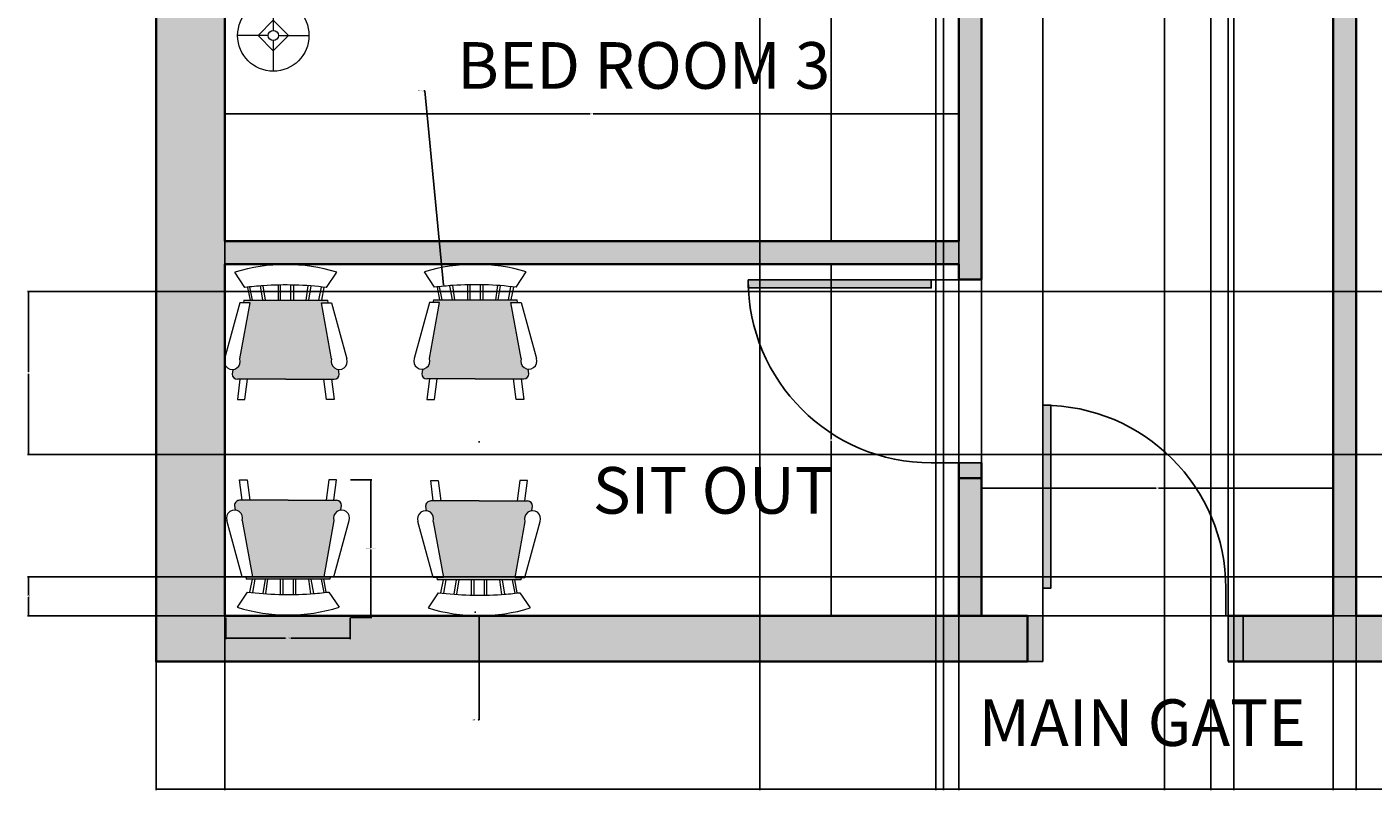
# Model space of a CAD drawing. Units: inches. Extents: x 1434 to 1845, y 1483 to 2014.
# Tile 1 of 11: x 1434 to 1698, y 1483 to 1633. Entities that reach past the tile are written whole.
import ezdxf

# ---------------------------------------------------------------- set-up
doc = ezdxf.new("R2010")
doc.units = ezdxf.units.IN
for name, color, linetype, lineweight in [('A-ANNO-DIMS', 2, 'Continuous', 18), ('A-ANNO-TEXT', 7, 'Continuous', 25), ('A-AREA-IDEN', 7, 'Continuous', 25), ('A-DOOR', 3, 'Continuous', 25), ('A-FURN', 9, 'Continuous', 18), ('A-FURN-PATT', 9, 'Continuous', 13), ('A-WALL', 7, 'Continuous', 35), ('A-WALL-PATT', 8, 'Continuous', 13), ('E-LITE', 2, 'Continuous', 18)]:
    doc.layers.add(name, color=color, linetype=linetype, lineweight=lineweight)
doc.layers.add('A-DOOR-PATT', color=39, linetype='Continuous', lineweight=13, true_color=0x58382b)
doc.styles.get("Standard").update_dxf_attribs({"font": 'arial.ttf'})
doc.dimstyles.get("Standard").update_dxf_attribs({"dimtxt": 0.18, "dimasz": 0.18, "dimexe": 0.18, "dimexo": 0.0625, "dimgap": 0.09, "dimtad": 0, "dimtih": 1, "dimtoh": 1, "dimdec": 4, "dimzin": 0, "dimdsep": 46, "dimtxsty": 'Standard', "dimcen": 0.09, "dimadec": 0, "dimazin": 0, "dimtfac": 1, "dimtdec": 4, "dimtofl": 0, "dimtmove": 0, "dimatfit": 3, "dimfxl": 1, "dimtolj": 1, "dimtzin": 0, "dimarcsym": 0})

# ---------------------------------------------------------------- blocks, each defined once
blk = doc.blocks.new('*U2')
for p, q in [((0, 0), (0, -6)), ((-40, 0), (-40, -6))]:
    blk.add_line(p, q)
blk.add_lwpolyline([(0, 0), (0, 40), (-1.75, 40), (-1.75, 0)], close=True)
blk.add_arc((0, 0), 40, 90, 180)
blk = doc.blocks.new('*U3')
for p, q in [((0, 0), (0, -6)), ((40, 0), (40, -6))]:
    blk.add_line(p, q)
blk.add_lwpolyline([(0, 0), (0, 40), (1.75, 40), (1.75, 0)], close=True)
blk.add_arc((0, 0), 40, 0, 90)
blk = doc.blocks.new('Chair - Rocking')
for p, q in [((-8, -4.5), (-10, -1.5)), ((8, -4.5), (10, -1.5)), ((-7.5, -4.5), (-7, -7)), ((-6.5, -7), (-7.02225, -4.43)), ((-4.5, -7), (-4.96674, -4.19951)), ((-4, -7), (-4.40532, -4.16272)), ((-1.5, -4.05012), (-1.5, -7)), ((-1, -7), (-1, -4.05012)), ((1, -7), (1, -4.04655)), ((1.5, -4.05012), (1.5, -7)), ((4, -7), (4.40187, -4.18694)), ((4.5, -7), (4.96761, -4.19437)), ((6.5, -7), (7, -4.4057)), ((7.5, -4.5), (7, -7)), ((-9, -7.5), (-12, -18.49999)), ((-7, -7.5), (-9, -7.5)), ((-9, -18.49999), (-7, -7.5)), ((-8.23428, -6.99939), (-8.3093, -7.47958)), ((-8.23041, -7), (8.23915, -7)), ((7, -7.5), (9, -7.5)), ((9, -18.49999), (7, -7.5)), ((8.31071, -7.48854), (8.23449, -7.00073)), ((9, -7.5), (12, -18.49999)), ((-10.36644, -20.64523), (-10.5, -21.49999)), ((10.5, -21.49999), (10.3575, -20.58798)), ((-9, -22.49999), (-9.5, -26.49999)), ((0, -22.49999), (-9.5, -22.49999)), ((-8, -26.49999), (-7.5, -22.49999)), ((0, -22.49999), (9.5, -22.49999)), ((8, -26.49999), (7.5, -22.49999)), ((9, -22.49999), (9.5, -26.49999)), ((-9.5, -26.49999), (-8, -26.49999)), ((9.5, -26.49999), (8, -26.49999))]:
    blk.add_line(p, q)
for centre, radius, start, end in [((0, -34.08333), 34.08333, 72.93847, 107.0615), ((0, -68.25004), 64.25, 93.92211, 97.15267), ((0, -68.25004), 64.25, 82.84733, 93.92211), ((-10.5, -18.99999), 1.58114, 161.5651, 18.43495), ((10.5, -18.99999), 1.58114, 161.5651, 18.43495), ((-9.5, -21.49999), 1, 180, 270), ((9.5, -21.49999), 1, 270, 0)]:
    blk.add_arc(centre, radius, start, end)
blk = doc.blocks.new('Lamp - Table')
for p, q in [((0, 7), (0, 1)), ((0, 3), (-3, 0)), ((3, 0), (0, 3)), ((-1, 0), (-7, 0)), ((-3, 0), (0, -3)), ((0, -3), (3, 0)), ((1, 0), (7, 0)), ((0, -1), (0, -7))]:
    blk.add_line(p, q)
for radius in [7, 1]:
    blk.add_circle((0, 0), radius)
blk = doc.blocks.new('*D30')
at = {"layer": 'A-ANNO-DIMS', "color": 0, "lineweight": -2, "transparency": 16777216}
for p, q in [((1497.66, 1544.02), (1501.83, 1544.02)), ((1501.65, 1543.84), (1501.65, 1530.7)), ((1501.65, 1517.2), (1501.65, 1530.34)), ((1497.66, 1517.02), (1501.83, 1517.02))]:
    blk.add_line(p, q, dxfattribs=at)
at = {"layer": 'A-ANNO-DIMS', "color": 0, "transparency": 16777216}
for points in [[(1501.62, 1543.84), (1501.68, 1543.84), (1501.65, 1544.02)], [(1501.62, 1517.2), (1501.68, 1517.2), (1501.65, 1517.02)]]:
    blk.add_solid(points, dxfattribs=at)
at = {"layer": 'Defpoints', "color": 0, "transparency": 16777216}
for p in [(1497.6, 1544.02), (1497.6, 1517.02), (1501.65, 1517.02)]:
    blk.add_point(p, dxfattribs=at)
at = {"layer": 'A-ANNO-DIMS', "color": 0, "transparency": 16777216, "insert": (1501.65, 1530.52), "char_height": 0.18, "attachment_point": 5}
blk.add_mtext('\\A1;ROCKER 27 TYP.', dxfattribs=at)
blk = doc.blocks.new('*D31')
at = {"layer": 'A-ANNO-DIMS', "color": 0, "lineweight": -2, "transparency": 16777216}
for p, q in [((1473.16, 1516.96), (1473.16, 1512.79)), ((1497.6, 1516.96), (1497.6, 1512.79)), ((1473.34, 1512.97), (1484.85, 1512.97)), ((1497.42, 1512.97), (1485.91, 1512.97))]:
    blk.add_line(p, q, dxfattribs=at)
at = {"layer": 'A-ANNO-DIMS', "color": 0, "transparency": 16777216}
for points in [[(1473.34, 1513), (1473.34, 1512.94), (1473.16, 1512.97)], [(1497.42, 1513), (1497.42, 1512.94), (1497.6, 1512.97)]]:
    blk.add_solid(points, dxfattribs=at)
at = {"layer": 'Defpoints', "color": 0, "transparency": 16777216}
for p in [(1473.16, 1517.02), (1497.6, 1517.02), (1473.16, 1512.97)]:
    blk.add_point(p, dxfattribs=at)
at = {"layer": 'A-ANNO-DIMS', "color": 0, "transparency": 16777216, "insert": (1485.38, 1512.97), "char_height": 0.18, "attachment_point": 5}
blk.add_mtext('\\A1;24 TYP.', dxfattribs=at)
blk = doc.blocks.new('*D54')
at = {"layer": 'A-ANNO-DIMS', "color": 0, "lineweight": -2, "transparency": 16777216}
for p, q in [((1459.47, 1508.29), (1459.47, 1483.15)), ((1819.47, 1508.29), (1819.47, 1483.15)), ((1459.65, 1483.33), (1639.19, 1483.33)), ((1819.29, 1483.33), (1639.76, 1483.33))]:
    blk.add_line(p, q, dxfattribs=at)
at = {"layer": 'A-ANNO-DIMS', "color": 0, "transparency": 16777216}
for points in [[(1459.65, 1483.36), (1459.65, 1483.3), (1459.47, 1483.33)], [(1819.29, 1483.36), (1819.29, 1483.3), (1819.47, 1483.33)]]:
    blk.add_solid(points, dxfattribs=at)
at = {"layer": 'Defpoints', "color": 0, "transparency": 16777216}
for p in [(1459.47, 1508.36), (1819.47, 1508.36), (1819.47, 1483.33)]:
    blk.add_point(p, dxfattribs=at)
at = {"layer": 'A-ANNO-DIMS', "color": 0, "transparency": 16777216, "insert": (1639.47, 1483.33), "char_height": 0.18, "attachment_point": 5}
blk.add_mtext('\\A1;360', dxfattribs=at)
blk = doc.blocks.new('*D56')
at = {"layer": 'A-ANNO-DIMS', "color": 0, "lineweight": -2, "transparency": 16777216}
for p, q in [((1472.97, 1974.79), (1472.97, 1483.15)), ((1612.47, 1974.79), (1612.47, 1483.15)), ((1473.15, 1483.33), (1542.34, 1483.33)), ((1612.29, 1483.33), (1543.11, 1483.33))]:
    blk.add_line(p, q, dxfattribs=at)
at = {"layer": 'A-ANNO-DIMS', "color": 0, "transparency": 16777216}
for points in [[(1473.15, 1483.36), (1473.15, 1483.3), (1472.97, 1483.33)], [(1612.29, 1483.36), (1612.29, 1483.3), (1612.47, 1483.33)]]:
    blk.add_solid(points, dxfattribs=at)
at = {"layer": 'Defpoints', "color": 0, "transparency": 16777216}
for p in [(1472.97, 1974.86), (1612.47, 1974.86), (1612.47, 1483.33)]:
    blk.add_point(p, dxfattribs=at)
at = {"layer": 'A-ANNO-DIMS', "color": 0, "transparency": 16777216, "insert": (1542.72, 1483.33), "char_height": 0.18, "attachment_point": 5}
blk.add_mtext('\\A1;139.5', dxfattribs=at)
blk = doc.blocks.new('*D57')
at = {"layer": 'A-ANNO-DIMS', "color": 0, "lineweight": -2, "transparency": 16777216}
for p, q in [((1616.97, 1974.79), (1616.97, 1483.15)), ((1666.47, 1974.79), (1666.47, 1483.15)), ((1617.15, 1483.33), (1641.4, 1483.33)), ((1666.29, 1483.33), (1642.05, 1483.33))]:
    blk.add_line(p, q, dxfattribs=at)
at = {"layer": 'A-ANNO-DIMS', "color": 0, "transparency": 16777216}
for points in [[(1617.15, 1483.36), (1617.15, 1483.3), (1616.97, 1483.33)], [(1666.29, 1483.36), (1666.29, 1483.3), (1666.47, 1483.33)]]:
    blk.add_solid(points, dxfattribs=at)
at = {"layer": 'Defpoints', "color": 0, "transparency": 16777216}
for p in [(1616.97, 1974.86), (1666.47, 1974.86), (1666.47, 1483.33)]:
    blk.add_point(p, dxfattribs=at)
at = {"layer": 'A-ANNO-DIMS', "color": 0, "transparency": 16777216, "insert": (1641.72, 1483.33), "char_height": 0.18, "attachment_point": 5}
blk.add_mtext('\\A1;49.5', dxfattribs=at)
blk = doc.blocks.new('*D58')
at = {"layer": 'A-ANNO-DIMS', "color": 0, "lineweight": -2, "transparency": 16777216}
for p, q in [((1670.97, 1974.79), (1670.97, 1483.15)), ((1810.47, 1974.79), (1810.47, 1483.15)), ((1671.15, 1483.33), (1740.34, 1483.33)), ((1810.29, 1483.33), (1741.11, 1483.33))]:
    blk.add_line(p, q, dxfattribs=at)
at = {"layer": 'A-ANNO-DIMS', "color": 0, "transparency": 16777216}
for points in [[(1671.15, 1483.36), (1671.15, 1483.3), (1670.97, 1483.33)], [(1810.29, 1483.36), (1810.29, 1483.3), (1810.47, 1483.33)]]:
    blk.add_solid(points, dxfattribs=at)
at = {"layer": 'Defpoints', "color": 0, "transparency": 16777216}
for p in [(1670.97, 1974.86), (1810.47, 1974.86), (1810.47, 1483.33)]:
    blk.add_point(p, dxfattribs=at)
at = {"layer": 'A-ANNO-DIMS', "color": 0, "transparency": 16777216, "insert": (1740.72, 1483.33), "char_height": 0.18, "attachment_point": 5}
blk.add_mtext('\\A1;139.5', dxfattribs=at)
blk = doc.blocks.new('*D64')
at = {"layer": 'A-ANNO-DIMS', "color": 0, "lineweight": -2, "transparency": 16777216}
for p, q in [((1472.97, 1590.92), (1472.97, 1616.06)), ((1473.15, 1615.88), (1544.69, 1615.88)), ((1616.79, 1615.88), (1545.25, 1615.88)), ((1616.97, 1590.92), (1616.97, 1616.06))]:
    blk.add_line(p, q, dxfattribs=at)
at = {"layer": 'A-ANNO-DIMS', "color": 0, "transparency": 16777216}
for points in [[(1473.15, 1615.91), (1473.15, 1615.85), (1472.97, 1615.88)], [(1616.79, 1615.91), (1616.79, 1615.85), (1616.97, 1615.88)]]:
    blk.add_solid(points, dxfattribs=at)
at = {"layer": 'Defpoints', "color": 0, "transparency": 16777216}
for p in [(1616.97, 1615.88), (1472.97, 1590.86), (1616.97, 1590.86)]:
    blk.add_point(p, dxfattribs=at)
at = {"layer": 'A-ANNO-DIMS', "color": 0, "transparency": 16777216, "insert": (1544.97, 1615.88), "char_height": 0.18, "attachment_point": 5}
blk.add_mtext('\\A1;144', dxfattribs=at)
blk = doc.blocks.new('*D65')
at = {"layer": 'A-ANNO-DIMS', "color": 0, "lineweight": -2, "transparency": 16777216}
for p, q in [((1616.91, 1730.36), (1591.77, 1730.36)), ((1591.95, 1730.18), (1591.95, 1660.79)), ((1591.95, 1591.04), (1591.95, 1660.42)), ((1616.91, 1590.86), (1591.77, 1590.86))]:
    blk.add_line(p, q, dxfattribs=at)
at = {"layer": 'A-ANNO-DIMS', "color": 0, "transparency": 16777216}
for points in [[(1591.92, 1730.18), (1591.98, 1730.18), (1591.95, 1730.36)], [(1591.92, 1591.04), (1591.98, 1591.04), (1591.95, 1590.86)]]:
    blk.add_solid(points, dxfattribs=at)
at = {"layer": 'Defpoints', "color": 0, "transparency": 16777216}
for p in [(1591.95, 1730.36), (1616.97, 1730.36), (1616.97, 1590.86)]:
    blk.add_point(p, dxfattribs=at)
at = {"layer": 'A-ANNO-DIMS', "color": 0, "transparency": 16777216, "insert": (1591.95, 1660.61), "char_height": 0.18, "attachment_point": 5}
blk.add_mtext('\\A1;139.5', dxfattribs=at)
blk = doc.blocks.new('*D66')
at = {"layer": 'A-ANNO-DIMS', "color": 0, "lineweight": -2, "transparency": 16777216}
for p, q in [((1616.91, 1586.36), (1591.77, 1586.36)), ((1591.95, 1586.18), (1591.95, 1552.04)), ((1591.95, 1517.54), (1591.95, 1551.67)), ((1616.91, 1517.36), (1591.77, 1517.36))]:
    blk.add_line(p, q, dxfattribs=at)
at = {"layer": 'A-ANNO-DIMS', "color": 0, "transparency": 16777216}
for points in [[(1591.92, 1586.18), (1591.98, 1586.18), (1591.95, 1586.36)], [(1591.92, 1517.54), (1591.98, 1517.54), (1591.95, 1517.36)]]:
    blk.add_solid(points, dxfattribs=at)
at = {"layer": 'Defpoints', "color": 0, "transparency": 16777216}
for p in [(1591.95, 1586.36), (1616.97, 1586.36), (1616.97, 1517.36)]:
    blk.add_point(p, dxfattribs=at)
at = {"layer": 'A-ANNO-DIMS', "color": 0, "transparency": 16777216, "insert": (1591.95, 1551.86), "char_height": 0.18, "attachment_point": 5}
blk.add_mtext('\\A1;69', dxfattribs=at)
blk = doc.blocks.new('*D67')
at = {"layer": 'A-ANNO-DIMS', "color": 0, "lineweight": -2, "transparency": 16777216}
for p, q in [((1694.97, 1517.42), (1694.97, 2013.56)), ((1695.15, 2013.38), (1752.34, 2013.38)), ((1810.29, 2013.38), (1753.11, 2013.38)), ((1810.47, 1517.42), (1810.47, 2013.56))]:
    blk.add_line(p, q, dxfattribs=at)
at = {"layer": 'A-ANNO-DIMS', "color": 0, "transparency": 16777216}
for points in [[(1695.15, 2013.41), (1695.15, 2013.35), (1694.97, 2013.38)], [(1810.29, 2013.41), (1810.29, 2013.35), (1810.47, 2013.38)]]:
    blk.add_solid(points, dxfattribs=at)
at = {"layer": 'Defpoints', "color": 0, "transparency": 16777216}
for p in [(1810.47, 2013.38), (1694.97, 1517.36), (1810.47, 1517.36)]:
    blk.add_point(p, dxfattribs=at)
at = {"layer": 'A-ANNO-DIMS', "color": 0, "transparency": 16777216, "insert": (1752.72, 2013.38), "char_height": 0.18, "attachment_point": 5}
blk.add_mtext('\\A1;115.5', dxfattribs=at)
blk = doc.blocks.new('*D70')
at = {"layer": 'A-ANNO-DIMS', "color": 0, "lineweight": -2, "transparency": 16777216}
for p, q in [((1621.47, 1517.42), (1621.47, 1542.56)), ((1621.65, 1542.38), (1655.75, 1542.38)), ((1690.29, 1542.38), (1656.19, 1542.38)), ((1690.47, 1517.42), (1690.47, 1542.56))]:
    blk.add_line(p, q, dxfattribs=at)
at = {"layer": 'A-ANNO-DIMS', "color": 0, "transparency": 16777216}
for points in [[(1621.65, 1542.41), (1621.65, 1542.35), (1621.47, 1542.38)], [(1690.29, 1542.41), (1690.29, 1542.35), (1690.47, 1542.38)]]:
    blk.add_solid(points, dxfattribs=at)
at = {"layer": 'Defpoints', "color": 0, "transparency": 16777216}
for p in [(1690.47, 1542.38), (1621.47, 1517.36), (1690.47, 1517.36)]:
    blk.add_point(p, dxfattribs=at)
at = {"layer": 'A-ANNO-DIMS', "color": 0, "transparency": 16777216, "insert": (1655.97, 1542.38), "char_height": 0.18, "attachment_point": 5}
blk.add_mtext('\\A1;69', dxfattribs=at)
blk = doc.blocks.new('*D71')
at = {"layer": 'A-ANNO-DIMS', "color": 0, "lineweight": -2, "transparency": 16777216}
for p, q in [((1633.47, 1508.42), (1633.47, 2013.56)), ((1633.65, 2013.38), (1651.25, 2013.38)), ((1669.64, 2013.38), (1652.04, 2013.38)), ((1669.82, 1508.42), (1669.82, 2013.56))]:
    blk.add_line(p, q, dxfattribs=at)
at = {"layer": 'A-ANNO-DIMS', "color": 0, "transparency": 16777216}
for points in [[(1633.65, 2013.41), (1633.65, 2013.35), (1633.47, 2013.38)], [(1669.64, 2013.41), (1669.64, 2013.35), (1669.82, 2013.38)]]:
    blk.add_solid(points, dxfattribs=at)
at = {"layer": 'Defpoints', "color": 0, "transparency": 16777216}
for p in [(1669.82, 2013.38), (1633.47, 1508.36), (1669.82, 1508.36)]:
    blk.add_point(p, dxfattribs=at)
at = {"layer": 'A-ANNO-DIMS', "color": 0, "transparency": 16777216, "insert": (1651.65, 2013.38), "char_height": 0.18, "attachment_point": 5}
blk.add_mtext('\\A1;36.35', dxfattribs=at)
blk = doc.blocks.new('*D72')
at = {"layer": 'A-ANNO-DIMS', "color": 0, "lineweight": -2, "transparency": 16777216}
for p, q in [((1621.47, 1517.42), (1621.47, 2013.56)), ((1621.65, 2013.38), (1627.26, 2013.38)), ((1633.29, 2013.38), (1627.68, 2013.38)), ((1633.47, 1517.42), (1633.47, 2013.56))]:
    blk.add_line(p, q, dxfattribs=at)
at = {"layer": 'A-ANNO-DIMS', "color": 0, "transparency": 16777216}
for points in [[(1621.65, 2013.41), (1621.65, 2013.35), (1621.47, 2013.38)], [(1633.29, 2013.41), (1633.29, 2013.35), (1633.47, 2013.38)]]:
    blk.add_solid(points, dxfattribs=at)
at = {"layer": 'Defpoints', "color": 0, "transparency": 16777216}
for p in [(1633.47, 2013.38), (1621.47, 1517.36), (1633.47, 1517.36)]:
    blk.add_point(p, dxfattribs=at)
at = {"layer": 'A-ANNO-DIMS', "color": 0, "transparency": 16777216, "insert": (1627.47, 2013.38), "char_height": 0.18, "attachment_point": 5}
blk.add_mtext('\\A1;12', dxfattribs=at)
blk = doc.blocks.new('*D73')
at = {"layer": 'A-ANNO-DIMS', "color": 0, "lineweight": -2, "transparency": 16777216}
for p, q in [((1577.97, 1730.29), (1577.97, 1483.15)), ((1613.97, 1730.29), (1613.97, 1483.15)), ((1578.15, 1483.33), (1595.76, 1483.33)), ((1613.79, 1483.33), (1596.19, 1483.33))]:
    blk.add_line(p, q, dxfattribs=at)
at = {"layer": 'A-ANNO-DIMS', "color": 0, "transparency": 16777216}
for points in [[(1578.15, 1483.36), (1578.15, 1483.3), (1577.97, 1483.33)], [(1613.79, 1483.36), (1613.79, 1483.3), (1613.97, 1483.33)]]:
    blk.add_solid(points, dxfattribs=at)
at = {"layer": 'Defpoints', "color": 0, "transparency": 16777216}
for p in [(1577.97, 1730.36), (1613.97, 1730.36), (1613.97, 1483.33)]:
    blk.add_point(p, dxfattribs=at)
at = {"layer": 'A-ANNO-DIMS', "color": 0, "transparency": 16777216, "insert": (1595.97, 1483.33), "char_height": 0.18, "attachment_point": 5}
blk.add_mtext('\\A1;36', dxfattribs=at)
blk = doc.blocks.new('*D81')
at = {"layer": 'A-ANNO-DIMS', "color": 0, "lineweight": -2, "transparency": 16777216}
for p, q in [((1690.47, 1730.29), (1690.47, 1483.15)), ((1694.97, 1730.29), (1694.97, 1483.15)), ((1690.65, 1483.33), (1692.47, 1483.33)), ((1694.79, 1483.33), (1692.98, 1483.33))]:
    blk.add_line(p, q, dxfattribs=at)
at = {"layer": 'A-ANNO-DIMS', "color": 0, "transparency": 16777216}
for points in [[(1690.65, 1483.36), (1690.65, 1483.3), (1690.47, 1483.33)], [(1694.79, 1483.36), (1694.79, 1483.3), (1694.97, 1483.33)]]:
    blk.add_solid(points, dxfattribs=at)
at = {"layer": 'Defpoints', "color": 0, "transparency": 16777216}
for p in [(1690.47, 1730.36), (1694.97, 1730.36), (1694.97, 1483.33)]:
    blk.add_point(p, dxfattribs=at)
at = {"layer": 'A-ANNO-DIMS', "color": 0, "transparency": 16777216, "insert": (1692.72, 1483.33), "char_height": 0.18, "attachment_point": 5}
blk.add_mtext('\\A1;4.5', dxfattribs=at)
blk = doc.blocks.new('*D82')
at = {"layer": 'A-ANNO-DIMS', "color": 0, "lineweight": -2, "transparency": 16777216}
for p, q in [((1704.55, 1524.96), (1704.55, 1483.15)), ((1694.97, 1517.29), (1694.97, 1483.15)), ((1695.15, 1483.33), (1699.37, 1483.33)), ((1704.37, 1483.33), (1700.16, 1483.33))]:
    blk.add_line(p, q, dxfattribs=at)
at = {"layer": 'A-ANNO-DIMS', "color": 0, "transparency": 16777216}
for points in [[(1695.15, 1483.36), (1695.15, 1483.3), (1694.97, 1483.33)], [(1704.37, 1483.36), (1704.37, 1483.3), (1704.55, 1483.33)]]:
    blk.add_solid(points, dxfattribs=at)
at = {"layer": 'Defpoints', "color": 0, "transparency": 16777216}
for p in [(1704.55, 1525.02), (1694.97, 1517.36), (1704.55, 1483.33)]:
    blk.add_point(p, dxfattribs=at)
at = {"layer": 'A-ANNO-DIMS', "color": 0, "transparency": 16777216, "insert": (1699.76, 1483.33), "char_height": 0.18, "attachment_point": 5}
blk.add_mtext('\\A1;9.576', dxfattribs=at)
blk = doc.blocks.new('*D83')
at = {"layer": 'A-ANNO-DIMS', "color": 0, "lineweight": -2, "transparency": 16777216}
for p, q in [((1704.49, 1525.02), (1434.27, 1525.02)), ((1434.45, 1524.84), (1434.45, 1521.37)), ((1434.45, 1517.54), (1434.45, 1521.01)), ((1694.91, 1517.36), (1434.27, 1517.36))]:
    blk.add_line(p, q, dxfattribs=at)
at = {"layer": 'A-ANNO-DIMS', "color": 0, "transparency": 16777216}
for points in [[(1434.42, 1524.84), (1434.48, 1524.84), (1434.45, 1525.02)], [(1434.42, 1517.54), (1434.48, 1517.54), (1434.45, 1517.36)]]:
    blk.add_solid(points, dxfattribs=at)
at = {"layer": 'Defpoints', "color": 0, "transparency": 16777216}
for p in [(1704.55, 1525.02), (1434.45, 1517.36), (1694.97, 1517.36)]:
    blk.add_point(p, dxfattribs=at)
at = {"layer": 'A-ANNO-DIMS', "color": 0, "transparency": 16777216, "insert": (1434.45, 1521.19), "char_height": 0.18, "attachment_point": 5}
blk.add_mtext('\\A1;7.664', dxfattribs=at)
blk = doc.blocks.new('*D84')
at = {"layer": 'A-ANNO-DIMS', "color": 0, "lineweight": -2, "transparency": 16777216}
for p, q in [((1704.49, 1581.02), (1434.27, 1581.02)), ((1434.45, 1580.84), (1434.45, 1565.2)), ((1434.45, 1549.2), (1434.45, 1564.84)), ((1704.49, 1549.02), (1434.27, 1549.02))]:
    blk.add_line(p, q, dxfattribs=at)
at = {"layer": 'A-ANNO-DIMS', "color": 0, "transparency": 16777216}
for points in [[(1434.42, 1580.84), (1434.48, 1580.84), (1434.45, 1581.02)], [(1434.42, 1549.2), (1434.48, 1549.2), (1434.45, 1549.02)]]:
    blk.add_solid(points, dxfattribs=at)
at = {"layer": 'Defpoints', "color": 0, "transparency": 16777216}
for p in [(1434.45, 1581.02), (1704.55, 1581.02), (1704.55, 1549.02)]:
    blk.add_point(p, dxfattribs=at)
at = {"layer": 'A-ANNO-DIMS', "color": 0, "transparency": 16777216, "insert": (1434.45, 1565.02), "char_height": 0.18, "attachment_point": 5}
blk.add_mtext('\\A1;32', dxfattribs=at)
blk = doc.blocks.new('*D86')
at = {"layer": 'A-ANNO-DIMS', "color": 0, "lineweight": -2, "transparency": 16777216}
for p, q in [((1657.38, 1854.66), (1657.38, 1483.15)), ((1666.47, 1854.79), (1666.47, 1483.15)), ((1657.56, 1483.33), (1661.53, 1483.33)), ((1666.29, 1483.33), (1662.32, 1483.33))]:
    blk.add_line(p, q, dxfattribs=at)
at = {"layer": 'A-ANNO-DIMS', "color": 0, "transparency": 16777216}
for points in [[(1657.56, 1483.36), (1657.56, 1483.3), (1657.38, 1483.33)], [(1666.29, 1483.36), (1666.29, 1483.3), (1666.47, 1483.33)]]:
    blk.add_solid(points, dxfattribs=at)
at = {"layer": 'Defpoints', "color": 0, "transparency": 16777216}
for p in [(1657.38, 1854.72), (1666.47, 1854.86), (1657.38, 1483.33)]:
    blk.add_point(p, dxfattribs=at)
at = {"layer": 'A-ANNO-DIMS', "color": 0, "transparency": 16777216, "insert": (1661.93, 1483.33), "char_height": 0.18, "attachment_point": 5}
blk.add_mtext('\\A1;9.096', dxfattribs=at)
blk = doc.blocks.new('*D98')
at = {"layer": 'A-ANNO-DIMS', "color": 0, "lineweight": -2, "transparency": 16777216}
for p, q in [((1512.02, 1620.39), (1512.2, 1620.39)), ((1512.2, 1620.39), (1515.91, 1582.2)), ((1522.03, 1518.07), (1522.21, 1518.07)), ((1522.12, 1517.98), (1522.12, 1518.16))]:
    blk.add_line(p, q, dxfattribs=at)
at = {"layer": 'A-ANNO-DIMS', "color": 0, "transparency": 16777216}
blk.add_solid([(1515.94, 1582.2), (1515.88, 1582.2), (1515.92, 1582.02)], dxfattribs=at)
at = {"layer": 'Defpoints', "color": 0, "transparency": 16777216}
for p in [(1515.92, 1582.02), (1522.12, 1518.07)]:
    blk.add_point(p, dxfattribs=at)
at = {"layer": 'A-ANNO-DIMS', "color": 0, "transparency": 16777216, "insert": (1511.35, 1620.39), "char_height": 0.18, "attachment_point": 5}
blk.add_mtext('\\A1;8X R64.25', dxfattribs=at)
blk = doc.blocks.new('*D99')
at = {"layer": 'A-ANNO-DIMS', "color": 0, "lineweight": -2, "transparency": 16777216}
for p, q in [((1522.78, 1551.46), (1522.96, 1551.46)), ((1522.87, 1551.37), (1522.87, 1551.55)), ((1522.87, 1496.93), (1522.87, 1517.2)), ((1522.69, 1496.93), (1522.87, 1496.93))]:
    blk.add_line(p, q, dxfattribs=at)
at = {"layer": 'A-ANNO-DIMS', "color": 0, "transparency": 16777216}
blk.add_solid([(1522.84, 1517.2), (1522.9, 1517.2), (1522.87, 1517.38)], dxfattribs=at)
at = {"layer": 'Defpoints', "color": 0, "transparency": 16777216}
for p in [(1522.87, 1551.46), (1522.87, 1517.38)]:
    blk.add_point(p, dxfattribs=at)
at = {"layer": 'A-ANNO-DIMS', "color": 0, "transparency": 16777216, "insert": (1522.01, 1496.93), "char_height": 0.18, "attachment_point": 5}
blk.add_mtext('\\A1;4X R34.08', dxfattribs=at)

msp = doc.modelspace()

# ---------------------------------------------------------------- hatches: boundary and pattern name
at = {"layer": 'A-DOOR-PATT'}
h = msp.add_hatch(color=256, dxfattribs=at)
h.dxf.hatch_style = 1
h.paths.add_polyline_path([(1611.5864, 1583.2737), (1575.6681, 1583.2737, 0.01094143), (1575.7025, 1581.7022), (1611.5864, 1581.7022)])
h.paths.add_polyline_path([(1621.4742, 1547.3553), (1616.9742, 1547.3553), (1616.9742, 1544.3553), (1621.4742, 1544.3553)])
h.paths.add_polyline_path([(1635.0456, 1558.627, 0.01094143), (1633.4742, 1558.6614), (1633.4742, 1522.7431), (1635.0456, 1522.7431)])
h.paths.add_polyline_path([(1633.4742, 1517.3553), (1630.4742, 1517.3553), (1630.4742, 1508.3553), (1633.4742, 1508.3553)])
h.paths.add_polyline_path([(1672.8212, 1517.3553), (1669.8212, 1517.3553), (1669.8212, 1508.3553), (1672.8212, 1508.3553)])
h.paths.add_polyline_path([(1613.8925, 1724.9676), (1612.3211, 1724.9676), (1612.3211, 1689.0836, 0.01094143), (1613.8925, 1689.0492)])
h.paths.add_polyline_path([(1789.3925, 1684.9726), (1753.4742, 1684.9726), (1753.4742, 1683.4011), (1789.3925, 1683.4011)])
h.paths.add_polyline_path([(1792.4742, 1679.5848), (1789.4742, 1679.5848), (1789.4742, 1675.0848), (1792.4742, 1675.0848)])
h.paths.add_polyline_path([(1563.5864, 1851.7737), (1527.6681, 1851.7737, 0.01094143), (1527.7025, 1850.2022), (1563.5864, 1850.2022)])
h.paths.add_polyline_path([(1609.3925, 1900.6614, 0.01094143), (1607.8211, 1900.627), (1607.8211, 1864.7431), (1609.3925, 1864.7431)])
h.paths.add_polyline_path([(1675.5456, 1900.627, 0.01094143), (1673.9742, 1900.6614), (1673.9742, 1864.7431), (1675.5456, 1864.7431)])
h.paths.add_polyline_path([(1751.2803, 1851.8553), (1715.3619, 1851.8553), (1715.3619, 1850.2839), (1751.2459, 1850.2839, 0.01094143)])
at = {"layer": 'A-FURN-PATT'}
h = msp.add_hatch(color=256, dxfattribs=at)
h.dxf.hatch_style = 1
h.paths.add_polyline_path([(1673.7517, 1809.0049), (1657.2829, 1809.0049), (1656.033, 1801.0049), (1675.0018, 1801.0049)])
h.paths.add_polyline_path([(1645.7517, 1809.0049), (1629.2829, 1809.0049), (1628.033, 1801.0049), (1647.0018, 1801.0049)])
h.paths.add_polyline_path([(1647.0018, 1765.0049), (1628.033, 1765.0049), (1629.2829, 1757.0049), (1645.7517, 1757.0049)])
h.paths.add_polyline_path([(1615.5173, 1792.4892), (1607.5173, 1791.2392), (1607.5173, 1774.7705), (1615.5173, 1773.5205)])
h.paths.add_polyline_path([(1675.0018, 1765.0049), (1656.033, 1765.0049), (1657.2829, 1757.0049), (1673.7517, 1757.0049)])
h.paths.add_polyline_path([(1695.5173, 1791.2392), (1687.5173, 1792.4892), (1687.5173, 1773.5205), (1695.5173, 1774.7705)])
h.paths.add_polyline_path([(1491.9292, 1578.7679), (1493.2417, 1578.7679), (1493.1636, 1579.2679), (1476.6949, 1579.2679), (1476.6168, 1578.7679), (1477.9292, 1578.7679), (1475.9292, 1567.7679, -0.4833507), (1474.5739, 1565.6934), (1474.4292, 1564.7679, 0.41421356), (1475.4292, 1563.7679), (1484.9292, 1563.7679), (1494.4292, 1563.7679, 0.41421356), (1495.4292, 1564.7679), (1495.2846, 1565.6934, -0.48335183), (1493.9292, 1567.7679)])
h.paths.add_polyline_path([(1529.1236, 1578.8204), (1530.4361, 1578.8204), (1530.3579, 1579.3204), (1513.8892, 1579.3204), (1513.8111, 1578.8204), (1515.1236, 1578.8204), (1513.1236, 1567.8204, -0.4833507), (1511.7682, 1565.7459), (1511.6236, 1564.8204, 0.41421356), (1512.6236, 1563.8204), (1522.1236, 1563.8204), (1531.6236, 1563.8204, 0.41421356), (1532.6236, 1564.8204), (1532.4789, 1565.7459, -0.48335183), (1531.1236, 1567.8204)])
h.paths.add_polyline_path([(1531.8672, 1535.8802, -0.4833507), (1533.2226, 1537.9547), (1533.3672, 1538.8802, 0.41421356), (1532.3672, 1539.8802), (1522.8672, 1539.8802), (1513.3672, 1539.8802, 0.41421356), (1512.3672, 1538.8802), (1512.5118, 1537.9547, -0.48335183), (1513.8672, 1535.8802), (1515.8672, 1524.8802), (1514.5547, 1524.8802), (1514.6329, 1524.3802), (1531.1016, 1524.3802), (1531.1797, 1524.8802), (1529.8672, 1524.8802)])
h.paths.add_polyline_path([(1494.3799, 1536.0192, -0.4833507), (1495.7353, 1538.0938), (1495.8799, 1539.0192, 0.41421356), (1494.8799, 1540.0192), (1485.3799, 1540.0192), (1475.8799, 1540.0192, 0.41421356), (1474.8799, 1539.0192), (1475.0245, 1538.0938, -0.48335183), (1476.3799, 1536.0192), (1478.3799, 1525.0193), (1477.0674, 1525.0193), (1477.1456, 1524.5193), (1493.6143, 1524.5193), (1493.6924, 1525.0193), (1492.3799, 1525.0193)])
at = {"layer": 'A-WALL-PATT'}
h = msp.add_hatch(color=256, dxfattribs=at)
h.dxf.hatch_style = 1
h.paths.add_polyline_path([(1472.9742, 1730.3553), (1577.9742, 1730.3553), (1577.9742, 1734.8553), (1573.4742, 1734.8553), (1573.4742, 1815.8553), (1568.9742, 1815.8553), (1568.9742, 1734.8553), (1472.9742, 1734.8553), (1472.9742, 1770.1951), (1459.9742, 1770.1951), (1459.9742, 1782.1951), (1459.9742, 1818.1951), (1472.9742, 1818.1951), (1472.9742, 1854.8553), (1568.9742, 1854.8553), (1568.9742, 1851.8553), (1573.4742, 1851.8553), (1573.4742, 1854.8553), (1573.4742, 1859.3553), (1472.9742, 1859.3553), (1472.9742, 1899.9369), (1459.9742, 1899.9369), (1459.9742, 1911.9369), (1459.9742, 1947.9369), (1472.9742, 1947.9369), (1472.9742, 1974.8553), (1513.9785, 1974.8553), (1513.9785, 1987.8553), (1561.9785, 1987.8553), (1561.9785, 1974.8553), (1612.4742, 1974.8553), (1612.4742, 1859.3553), (1609.4742, 1859.3553), (1609.4742, 1854.8553), (1616.9742, 1854.8553), (1616.9742, 1910.3553), (1625.153, 1910.3553), (1625.153, 1914.8553), (1616.9742, 1914.8553), (1616.9742, 1988.3553), (1459.4742, 1988.3553), (1459.4742, 1508.3553), (1630.4742, 1508.3553), (1630.4742, 1517.3553), (1472.9742, 1517.3553), (1472.9742, 1586.3553), (1616.9742, 1586.3553), (1616.9742, 1583.3553), (1621.4742, 1583.3553), (1621.4742, 1586.3553), (1621.4742, 1734.8553), (1616.9742, 1734.8553), (1613.9742, 1734.8553), (1613.9742, 1730.3553), (1616.9742, 1730.3553), (1616.9742, 1590.8553), (1472.9742, 1590.8553), (1472.9742, 1635.7299), (1459.9742, 1635.7299), (1459.9742, 1647.7299), (1459.9742, 1683.7299), (1472.9742, 1683.7299)])
h.paths.add_polyline_path([(1819.4742, 1773.1667), (1810.4742, 1773.1667), (1810.4742, 1734.8553), (1714.4742, 1734.8553), (1714.4742, 1815.8553), (1709.9742, 1815.8553), (1709.9742, 1730.3553), (1745.9742, 1730.3553), (1745.9742, 1675.0848), (1753.4742, 1675.0848), (1753.4742, 1679.5848), (1750.4742, 1679.5848), (1750.4742, 1730.3553), (1810.4742, 1730.3553), (1810.4742, 1679.5848), (1792.4742, 1679.5848), (1792.4742, 1675.0848), (1810.4742, 1675.0848), (1810.4742, 1517.3553), (1775.1129, 1517.3553), (1775.1129, 1508.3553), (1819.4742, 1508.3553)])
h.paths.add_polyline_path([(1739.1129, 1517.3553), (1694.9742, 1517.3553), (1694.9742, 1730.3553), (1690.4742, 1730.3553), (1690.4742, 1517.3553), (1678.4742, 1517.3553), (1675.4742, 1517.3553), (1672.8212, 1517.3553), (1672.8212, 1508.3553), (1678.4742, 1508.3553), (1739.1129, 1508.3553)])
h.paths.add_polyline_path([(1735.6549, 1987.8553), (1783.6549, 1987.8553), (1783.6549, 1974.8553), (1810.4742, 1974.8553), (1810.4742, 1859.3553), (1709.9742, 1859.3553), (1709.9742, 1854.8553), (1709.9742, 1851.8553), (1714.4742, 1851.8553), (1714.4742, 1854.8553), (1810.4742, 1854.8553), (1810.4742, 1809.1667), (1819.4742, 1809.1667), (1819.4742, 1988.3553), (1666.4742, 1988.3553), (1666.4742, 1914.8553), (1661.1087, 1914.8553), (1661.1087, 1910.3553), (1666.4742, 1910.3553), (1666.4742, 1854.8553), (1673.9742, 1854.8553), (1673.9742, 1859.3553), (1670.9742, 1859.3553), (1670.9742, 1974.8553), (1735.6549, 1974.8553)])
h = msp.add_hatch(color=256, dxfattribs=at)
h.dxf.hatch_style = 1
h.paths.add_polyline_path([(1621.4742, 1544.3553), (1616.9742, 1544.3553), (1616.9742, 1517.3553), (1621.4742, 1517.3553)])

# ---------------------------------------------------------------- linework, layer by layer
at = {"layer": 'A-DOOR'}
for p, q in [((1621.4742, 1547.3553), (1616.9742, 1547.3553)), ((1630.4742, 1517.3553), (1633.4742, 1517.3553)), ((1633.4742, 1508.3553), (1633.4742, 1517.3553)), ((1669.8212, 1517.3553), (1669.8212, 1508.3553)), ((1672.8212, 1517.3553), (1672.8212, 1508.3553)), ((1630.4742, 1508.3553), (1633.4742, 1508.3553))]:
    msp.add_line(p, q, dxfattribs=at)
at = {"layer": 'A-WALL'}
for p, q in [((1621.4742, 1734.8553), (1621.4742, 1586.3553)), ((1472.9742, 1730.3553), (1472.9742, 1590.8553)), ((1616.9742, 1730.3553), (1616.9742, 1590.8553)), ((1690.4742, 1517.3553), (1690.4742, 1730.3553)), ((1694.9742, 1517.3553), (1694.9742, 1730.3553)), ((1616.9742, 1590.8553), (1472.9742, 1590.8553)), ((1616.9742, 1586.3553), (1472.9742, 1586.3553)), ((1472.9742, 1586.3553), (1472.9742, 1517.3553)), ((1616.9742, 1586.3553), (1616.9742, 1583.3553)), ((1621.4742, 1586.3553), (1621.4742, 1583.3553)), ((1621.4742, 1583.3553), (1616.9742, 1583.3553)), ((1616.9742, 1547.3553), (1616.9742, 1517.3553)), ((1621.4742, 1547.3553), (1621.4742, 1517.3553)), ((1621.4742, 1544.3553), (1616.9742, 1544.3553)), ((1472.9742, 1517.3553), (1630.4742, 1517.3553)), ((1630.4742, 1508.3553), (1630.4742, 1517.3553)), ((1675.4742, 1517.3553), (1669.8212, 1517.3553)), ((1678.4742, 1517.3553), (1675.4742, 1517.3553)), ((1678.4742, 1517.3553), (1690.4742, 1517.3553)), ((1694.9742, 1517.3553), (1810.4742, 1517.3553)), ((1678.4742, 1508.3553), (1669.8212, 1508.3553))]:
    msp.add_line(p, q, dxfattribs=at)
msp.add_lwpolyline([(1678.4742, 1508.3553), (1819.4742, 1508.3553), (1819.4742, 1988.3553), (1459.4742, 1988.3553), (1459.4742, 1508.3553), (1630.4742, 1508.3553)], dxfattribs=at)

# ---------------------------------------------------------------- block references
at = {"layer": 'A-DOOR', "xscale": 0.8979587755198419, "yscale": 0.8979587755198419, "zscale": 0.8979587755198419, "rotation": 90}
msp.add_blockref('*U2', (1611.5864, 1583.2737), dxfattribs=at)
at = {"layer": 'A-DOOR', "xscale": 0.8979587755198419, "yscale": 0.8979587755198419, "zscale": 0.8979587755198419}
msp.add_blockref('*U3', (1633.4742, 1522.7431), dxfattribs=at)
at = {"layer": 'A-FURN'}
for p in [(1484.9292, 1586.2679), (1522.1236, 1586.3204)]:
    msp.add_blockref('Chair - Rocking', p, dxfattribs=at)
at = {"layer": 'A-FURN', "rotation": 180}
for p in [(1485.3799, 1517.5193), (1522.8672, 1517.3802)]:
    msp.add_blockref('Chair - Rocking', p, dxfattribs=at)
at = {"layer": 'E-LITE'}
msp.add_blockref('Lamp - Table', (1482.4912, 1631.214), dxfattribs=at)

# ---------------------------------------------------------------- texts
at = {"layer": 'A-ANNO-TEXT'}
msp.add_text('MAIN GATE ', height=9.14668, dxfattribs=at).set_placement((1620.861, 1491.8092))
at = {"layer": 'A-AREA-IDEN'}
for s, height, p in [('BED ROOM 3 ', 9.146682, (1518.5474, 1620.7742)), ('SIT OUT ', 9.14668, (1545.1729, 1537.3883))]:
    msp.add_text(s, height=height, dxfattribs=at).set_placement(p)

# ---------------------------------------------------------------- dimensions: what is measured, and where the dimension line sits
at = {"layer": 'A-ANNO-DIMS'}
for base, p1, p2, override, picture, middle in [((1633.4742, 2013.3803), (1621.4742, 1517.3553), (1633.4742, 1517.3553), {"dimdec": 0, "dimlfac": 1, "dimrnd": 0, "dimzin": 0, "dimdsep": 46, "dimlunit": 2}, '*D72', (1627.4742, 2013.3803)), ((1669.8212, 2013.3803), (1633.4742, 1508.3553), (1669.8212, 1508.3553), {"dimdec": 2, "dimlfac": 1, "dimrnd": 0, "dimzin": 0, "dimdsep": 46, "dimlunit": 2}, '*D71', (1651.6477, 2013.3803)), ((1810.4742, 2013.3803), (1694.9742, 1517.3553), (1810.4742, 1517.3553), {"dimdec": 1, "dimlfac": 1, "dimrnd": 0, "dimzin": 0, "dimdsep": 46, "dimlunit": 2}, '*D67', (1752.7242, 2013.3803)), ((1612.4742, 1483.3303), (1472.9742, 1974.8553), (1612.4742, 1974.8553), {"dimdec": 1, "dimlfac": 1, "dimrnd": 0, "dimzin": 0, "dimdsep": 46, "dimlunit": 2}, '*D56', (1542.7242, 1483.3303)), ((1666.4742, 1483.3303), (1616.9742, 1974.8553), (1666.4742, 1974.8553), {"dimdec": 1, "dimlfac": 1, "dimrnd": 0, "dimzin": 0, "dimdsep": 46, "dimlunit": 2}, '*D57', (1641.7242, 1483.3303)), ((1810.4742, 1483.3303), (1670.9742, 1974.8553), (1810.4742, 1974.8553), {"dimdec": 1, "dimlfac": 1, "dimrnd": 0, "dimzin": 0, "dimdsep": 46, "dimlunit": 2}, '*D58', (1740.7242, 1483.3303)), ((1657.3781, 1483.3303), (1666.4742, 1854.8553), (1657.3781, 1854.7205), {"dimdec": 3, "dimlfac": 1, "dimrnd": 0, "dimzin": 0, "dimdsep": 46, "dimlunit": 2}, '*D86', (1661.9261, 1483.3303)), ((1613.9742, 1483.3303), (1577.9742, 1730.3553), (1613.9742, 1730.3553), {"dimdec": 0, "dimlfac": 1, "dimrnd": 0, "dimzin": 0, "dimdsep": 46, "dimlunit": 2}, '*D73', (1595.9742, 1483.3303)), ((1694.9742, 1483.3303), (1690.4742, 1730.3553), (1694.9742, 1730.3553), {"dimdec": 1, "dimlfac": 1, "dimrnd": 0, "dimzin": 0, "dimdsep": 46, "dimlunit": 2}, '*D81', (1692.7242, 1483.3303)), ((1616.9742, 1615.8803), (1472.9742, 1590.8553), (1616.9742, 1590.8553), {"dimdec": 0, "dimlfac": 1, "dimrnd": 0, "dimzin": 0, "dimdsep": 46, "dimlunit": 2}, '*D64', (1544.9742, 1615.8803)), ((1690.4742, 1542.3803), (1621.4742, 1517.3553), (1690.4742, 1517.3553), {"dimdec": 0, "dimlfac": 1, "dimrnd": 0, "dimzin": 0, "dimdsep": 46, "dimlunit": 2}, '*D70', (1655.9742, 1542.3803)), ((1704.5505, 1483.3303), (1694.9742, 1517.3553), (1704.5505, 1525.0191), {"dimdec": 3, "dimlfac": 1, "dimrnd": 0, "dimzin": 0, "dimdsep": 46, "dimlunit": 2}, '*D82', (1699.7623, 1483.3303)), ((1819.4742, 1483.3303), (1459.4742, 1508.3553), (1819.4742, 1508.3553), {"dimdec": 0, "dimlfac": 1, "dimrnd": 0, "dimzin": 0, "dimdsep": 46, "dimlunit": 2}, '*D54', (1639.4742, 1483.3303))]:
    dim = msp.add_linear_dim(base=base, p1=p1, p2=p2, dimstyle='Standard', override=override, dxfattribs=at)
    dim.commit()
    dim.dimension.update_dxf_attribs({"geometry": picture, "text_midpoint": middle})
for base, p1, p2, override, picture, middle in [((1591.9492, 1730.3553), (1616.9742, 1590.8553), (1616.9742, 1730.3553), {"dimdec": 1, "dimlfac": 1, "dimrnd": 0, "dimzin": 0, "dimdsep": 46, "dimlunit": 2}, '*D65', (1591.9492, 1660.6053)), ((1591.9492, 1586.3553), (1616.9742, 1517.3553), (1616.9742, 1586.3553), {"dimdec": 0, "dimlfac": 1, "dimrnd": 0, "dimzin": 0, "dimdsep": 46, "dimlunit": 2}, '*D66', (1591.9492, 1551.8553)), ((1434.4492, 1581.019), (1704.5505, 1549.0191), (1704.5505, 1581.019), {"dimdec": 0, "dimlfac": 1, "dimrnd": 0, "dimzin": 0, "dimdsep": 46, "dimlunit": 2}, '*D84', (1434.4492, 1565.0191)), ((1434.4492, 1517.3553), (1704.5505, 1525.0191), (1694.9742, 1517.3553), {"dimdec": 3, "dimlfac": 1, "dimrnd": 0, "dimzin": 0, "dimdsep": 46, "dimlunit": 2}, '*D83', (1434.4492, 1521.1872))]:
    dim = msp.add_linear_dim(base=base, p1=p1, p2=p2, angle=90, dimstyle='Standard', override=override, dxfattribs=at)
    dim.commit()
    dim.dimension.update_dxf_attribs({"geometry": picture, "text_midpoint": middle})
for center, mpoint, text, picture, middle in [((1522.1236, 1518.0704), (1515.924, 1582.0206), '8X <>', '*D98', (1511.3503, 1620.3907)), ((1522.8672, 1551.4636), (1522.867, 1517.3802), '4X <>', '*D99', (1522.0098, 1496.9302))]:
    dim = msp.add_radius_dim(center=center, mpoint=mpoint, text=text, dimstyle='Standard', override={"dimdec": 2, "dimlfac": 1, "dimrnd": 0, "dimzin": 0, "dimdsep": 46, "dimlunit": 2}, dxfattribs=at)
    dim.commit()
    dim.dimension.update_dxf_attribs({"geometry": picture, "text_midpoint": middle, "dimtype": 164})
for base, p1, p2, angle, text, picture, middle in [((1501.6475, 1517.0193), (1497.5975, 1544.0192), (1497.5975, 1517.0193), 270, 'ROCKER <> TYP.', '*D30', (1501.6475, 1530.5193)), ((1473.1624, 1512.9693), (1497.5975, 1517.0193), (1473.1624, 1517.0193), 180, '<> TYP.', '*D31', (1485.3799, 1512.9693))]:
    dim = msp.add_linear_dim(base=base, p1=p1, p2=p2, angle=angle, text=text, dimstyle='Standard', override={"dimdec": 0, "dimlfac": 1, "dimrnd": 0, "dimzin": 0, "dimdsep": 46, "dimlunit": 2}, dxfattribs=at)
    dim.commit()
    dim.dimension.update_dxf_attribs({"geometry": picture, "text_midpoint": middle})

doc.saveas('drawing.dxf')
